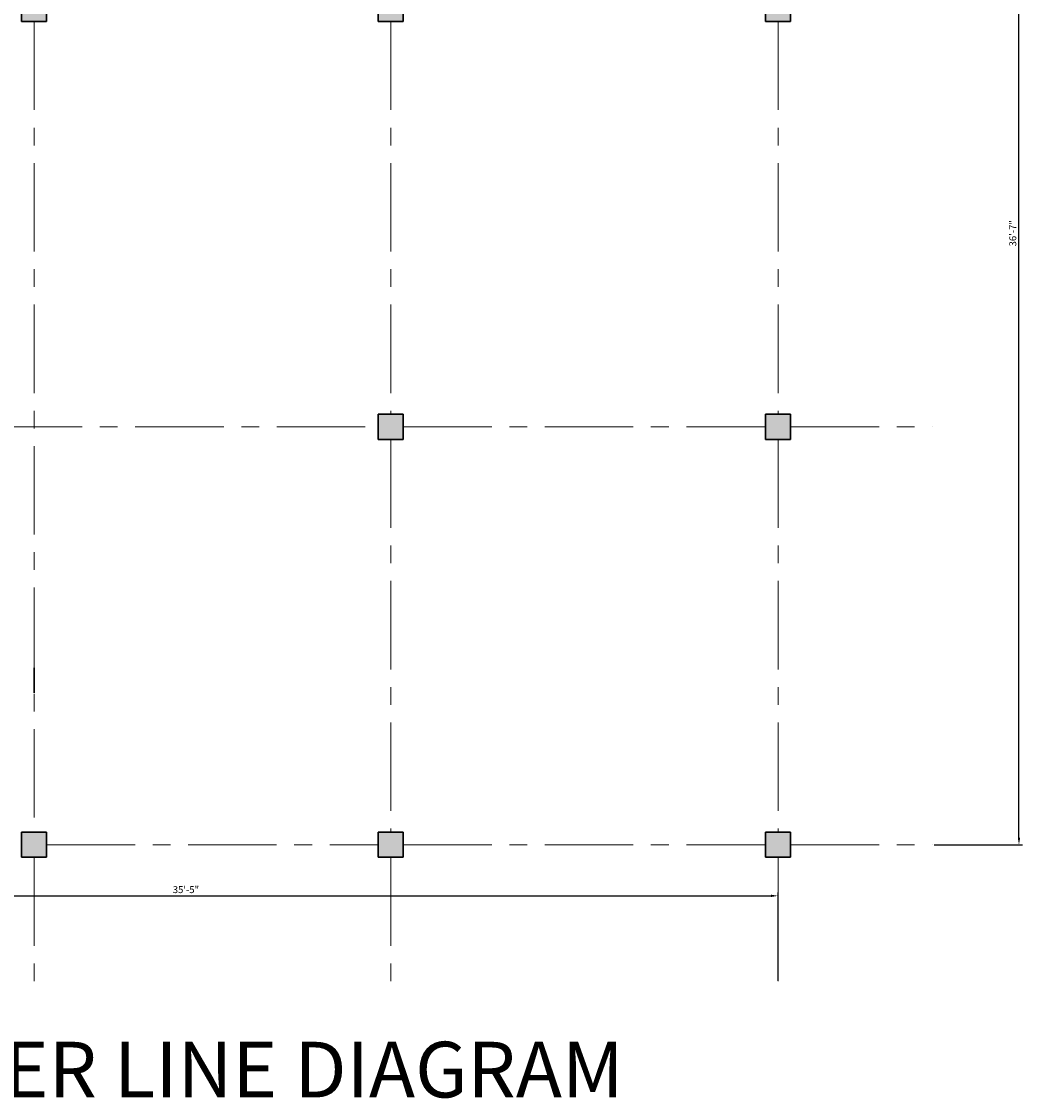
# Model space of a CAD drawing. Units: inches. Extents: x 4878 to 9282, y 5367 to 6617.
# Tile 13 of 14: x 8923 to 9282, y 5977 to 6364. Entities that reach past the tile are written whole.
import ezdxf

# ---------------------------------------------------------------- set-up
doc = ezdxf.new("R2010")
doc.units = ezdxf.units.IN
doc.linetypes.add('CENTER', pattern=[50.8, 31.75, -6.35, 6.35, -6.35])
for name, color, linetype, lineweight in [('A-ANNO-DIMS', 2, 'Continuous', 18), ('A-ANNO-TITL', 3, 'Continuous', 30), ('S-COLS', 1, 'Continuous', 30), ('S-COLS-PATT', 1, 'Continuous', 13), ('S-GRID', 4, 'CENTER', 13)]:
    doc.layers.add(name, color=color, linetype=linetype, lineweight=lineweight)
doc.styles.get("Standard").update_dxf_attribs({"font": 'arial.ttf'})
doc.dimstyles.new('ISO-25', dxfattribs={"dimtxt": 2.5, "dimasz": 2.5, "dimexe": 1.25, "dimexo": 0.625, "dimtad": 1, "dimdec": 0, "dimlunit": 3, "dimtxsty": 'Standard', "dimcen": 2.5, "dimadec": 0, "dimazin": 0, "dimtfac": 1, "dimtdec": 0, "dimtmove": 0, "dimatfit": 3, "dimfxl": 1, "dimarcsym": 0})

# ---------------------------------------------------------------- blocks, each defined once
blk = doc.blocks.new('COLUMN-9X9')
for p, q in [((0, 9), (9, 9)), ((0, 0), (0, 9)), ((9, 9), (9, 0)), ((0, 0), (9, 0))]:
    blk.add_line(p, q)
blk = doc.blocks.new('*D83')
at = {"layer": 'A-ANNO-DIMS', "color": 0, "lineweight": -2, "transparency": 16777216}
for p, q in [((8769.46, 6019.46), (8769.46, 6051.18)), ((9194.46, 6019.46), (9194.46, 6051.18)), ((8771.96, 6049.93), (9191.96, 6049.93))]:
    blk.add_line(p, q, dxfattribs=at)
at = {"layer": 'A-ANNO-DIMS', "color": 0, "transparency": 16777216}
for points in [[(8771.96, 6050.35), (8771.96, 6049.51), (8769.46, 6049.93)], [(9191.96, 6050.35), (9191.96, 6049.51), (9194.46, 6049.93)]]:
    blk.add_solid(points, dxfattribs=at)
at = {"layer": 'Defpoints', "color": 0, "transparency": 16777216}
for p in [(9194.46, 6049.93), (8769.46, 6018.83), (9194.46, 6018.83)]:
    blk.add_point(p, dxfattribs=at)
at = {"layer": 'A-ANNO-DIMS', "color": 0, "transparency": 16777216, "insert": (8981.96, 6051.83), "char_height": 2.5, "attachment_point": 5}
blk.add_mtext('35\'-5"', dxfattribs=at)
blk = doc.blocks.new('*D87')
at = {"layer": 'A-ANNO-DIMS', "color": 0, "lineweight": -2, "transparency": 16777216}
for p, q in [((9250.46, 6507.27), (9282.18, 6507.27)), ((9280.93, 6070.77), (9280.93, 6504.77)), ((9250.46, 6068.27), (9282.18, 6068.27))]:
    blk.add_line(p, q, dxfattribs=at)
at = {"layer": 'A-ANNO-DIMS', "color": 0, "transparency": 16777216}
for points in [[(9280.52, 6504.77), (9281.35, 6504.77), (9280.93, 6507.27)], [(9280.52, 6070.77), (9281.35, 6070.77), (9280.93, 6068.27)]]:
    blk.add_solid(points, dxfattribs=at)
at = {"layer": 'Defpoints', "color": 0, "transparency": 16777216}
for p in [(9249.83, 6507.27), (9280.93, 6507.27), (9249.83, 6068.27)]:
    blk.add_point(p, dxfattribs=at)
at = {"layer": 'A-ANNO-DIMS', "color": 0, "transparency": 16777216, "insert": (9279.03, 6287.77), "char_height": 2.5, "attachment_point": 5, "rotation": 90}
blk.add_mtext('36\'-7"', dxfattribs=at)

msp = doc.modelspace()

# ---------------------------------------------------------------- hatches: boundary and pattern name
at = {"layer": 'S-COLS-PATT'}
h = msp.add_hatch(color=256, dxfattribs=at)
h.dxf.hatch_style = 1
h.paths.add_polyline_path([(8931.96, 6072.77), (8922.96, 6072.77), (8922.96, 6063.77), (8931.96, 6063.77)])
h.paths.add_polyline_path([(9059.96, 6072.77), (9050.96, 6072.77), (9050.96, 6063.77), (9059.96, 6063.77)])
h.paths.add_polyline_path([(9198.96, 6072.77), (9189.96, 6072.77), (9189.96, 6063.77), (9198.96, 6063.77)])
h.paths.add_polyline_path([(9198.96, 6222.77), (9189.96, 6222.77), (9189.96, 6213.77), (9198.96, 6213.77)])
h.paths.add_polyline_path([(9059.96, 6222.77), (9050.96, 6222.77), (9050.96, 6213.77), (9059.96, 6213.77)])
h.paths.add_polyline_path([(8912.96, 6222.77), (8903.96, 6222.77), (8903.96, 6213.77), (8912.96, 6213.77)])
h.paths.add_polyline_path([(8773.96, 6222.77), (8764.96, 6222.77), (8764.96, 6213.77), (8773.96, 6213.77)])
h.paths.add_polyline_path([(8773.96, 6372.77), (8764.96, 6372.77), (8764.96, 6363.77), (8773.96, 6363.77)])
h.paths.add_polyline_path([(8931.96, 6372.77), (8922.96, 6372.77), (8922.96, 6363.77), (8931.96, 6363.77)])
h.paths.add_polyline_path([(9059.96, 6372.77), (9050.96, 6372.77), (9050.96, 6363.77), (9059.96, 6363.77)])
h.paths.add_polyline_path([(9198.96, 6372.77), (9189.96, 6372.77), (9189.96, 6363.77), (9198.96, 6363.77)])
h.paths.add_polyline_path([(9198.96, 6511.77), (9189.96, 6511.77), (9189.96, 6502.77), (9198.96, 6502.77)])
h.paths.add_polyline_path([(9059.96, 6511.77), (9050.96, 6511.77), (9050.96, 6502.77), (9059.96, 6502.77)])
h.paths.add_polyline_path([(8912.96, 6511.77), (8903.96, 6511.77), (8903.96, 6502.77), (8912.96, 6502.77)])
h.paths.add_polyline_path([(8773.96, 6511.77), (8764.96, 6511.77), (8764.96, 6502.77), (8773.96, 6502.77)])

# ---------------------------------------------------------------- linework, layer by layer
at = {"layer": 'S-COLS'}
msp.add_line((8927.46, 6131.77), (8927.46, 6122.77), dxfattribs=at)
at = {"layer": 'S-GRID'}
for p, q in [((8927.46, 6363.77), (8927.46, 6072.77)), ((9055.46, 6363.77), (9055.46, 6222.77)), ((9194.46, 6363.77), (9194.46, 6222.77)), ((8912.96, 6218.27), (9050.96, 6218.27)), ((9059.96, 6218.27), (9189.96, 6218.27)), ((9198.96, 6218.27), (9249.83, 6218.27)), ((9055.46, 6213.77), (9055.46, 6072.77)), ((9194.46, 6213.77), (9194.46, 6072.77)), ((8773.96, 6068.27), (8922.96, 6068.27)), ((8931.96, 6068.27), (9050.96, 6068.27)), ((9059.96, 6068.27), (9189.96, 6068.27)), ((9198.96, 6068.27), (9249.83, 6068.27)), ((8927.46, 6063.77), (8927.46, 6018.83)), ((9055.46, 6063.77), (9055.46, 6018.83)), ((9194.46, 6063.77), (9194.46, 6018.83))]:
    msp.add_line(p, q, dxfattribs=at)

# ---------------------------------------------------------------- block references
at = {"layer": 'S-COLS'}
for p in [(8922.96, 6363.77), (9050.96, 6363.77), (9189.96, 6363.77), (9050.96, 6213.77), (9189.96, 6213.77), (8922.96, 6063.77), (9050.96, 6063.77), (9189.96, 6063.77)]:
    msp.add_blockref('COLUMN-9X9', p, dxfattribs=at)

# ---------------------------------------------------------------- texts
at = {"layer": 'A-ANNO-TITL', "insert": (8847.07, 5997.54), "char_height": 20, "attachment_point": 1}
msp.add_mtext_dynamic_manual_height_columns('CENTER LINE DIAGRAM', width=599.8964, gutter_width=12.5, heights=[0], dxfattribs=at)

# ---------------------------------------------------------------- dimensions: what is measured, and where the dimension line sits
at = {"layer": 'A-ANNO-DIMS'}
dim = msp.add_linear_dim(base=(9280.93, 6507.27), p1=(9249.83, 6068.27), p2=(9249.83, 6507.27), angle=90, dimstyle='ISO-25', override={"dimdec": 1, "dimlfac": 1, "dimrnd": 0, "dimzin": 1, "dimdsep": 46, "dimlunit": 4, "dimfrac": 2}, dxfattribs=at)
dim.commit()
dim.dimension.update_dxf_attribs({"geometry": '*D87', "text_midpoint": (9279.03, 6287.77)})
dim = msp.add_linear_dim(base=(9194.46, 6049.93), p1=(8769.46, 6018.83), p2=(9194.46, 6018.83), dimstyle='ISO-25', override={"dimdec": 1, "dimlfac": 1, "dimrnd": 0, "dimzin": 1, "dimdsep": 46, "dimlunit": 4, "dimfrac": 2}, dxfattribs=at)
dim.commit()
dim.dimension.update_dxf_attribs({"geometry": '*D83', "text_midpoint": (8981.96, 6051.83)})

doc.saveas('drawing.dxf')
